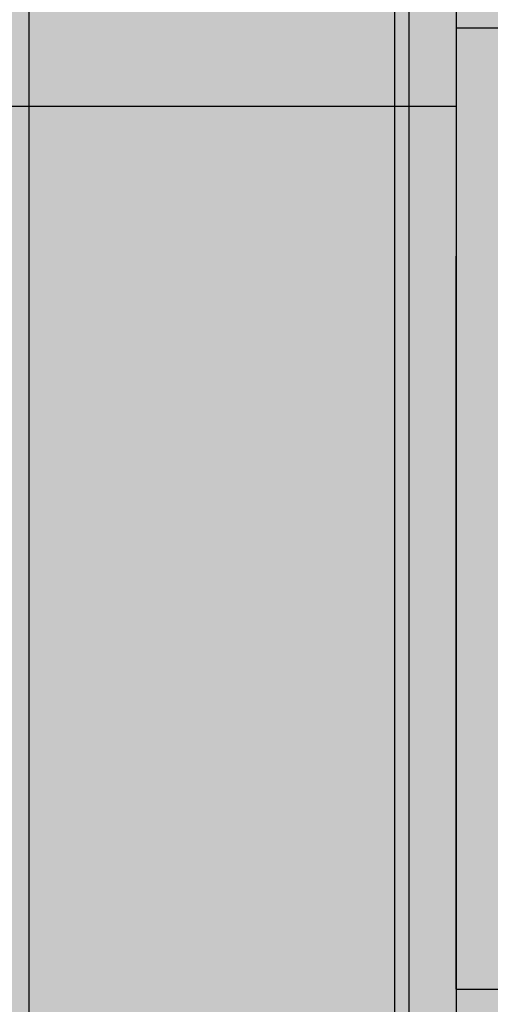
# Model space of a CAD drawing. Units: millimetres. Extents: x 131 to 845, y -20 to 1043.
# Tile 3 of 11: x 368 to 467, y 95 to 302. Entities that reach past the tile are written whole.
import ezdxf

# ---------------------------------------------------------------- set-up
doc = ezdxf.new("R2010")
doc.units = ezdxf.units.MM
doc.header["$MEASUREMENT"] = 0
for name, color, linetype, lineweight in [('A-ANNO-DIMS', 2, 'Continuous', 18), ('A-ELEV', 7, 'Continuous', 25), ('A-ELEV-PATT', 7, 'Continuous', 13), ('A-GLAZ-PATT', 143, 'Continuous', 13), ('A-WALL-PATT', 131, 'Continuous', 13)]:
    doc.layers.add(name, color=color, linetype=linetype, lineweight=lineweight)
doc.styles.get("Standard").update_dxf_attribs({"font": 'arial.ttf'})
doc.dimstyles.get("Standard").update_dxf_attribs({"dimtxt": 15, "dimasz": 10, "dimexe": 0.18, "dimexo": 0.0625, "dimgap": 5, "dimtad": 0, "dimtih": 1, "dimtoh": 1, "dimdec": 0, "dimzin": 0, "dimdsep": 46, "dimtxsty": 'Standard', "dimcen": 5, "dimadec": 0, "dimazin": 0, "dimtfac": 1, "dimtdec": 0, "dimtofl": 0, "dimtmove": 0, "dimatfit": 3, "dimfxl": 1, "dimtolj": 1, "dimtzin": 0, "dimarcsym": 0})

# ---------------------------------------------------------------- blocks, each defined once
blk = doc.blocks.new('*U5')
blk.add_line((0, 90), (0, 0))
blk = doc.blocks.new('*U6')
at = {"layer": 'A-ELEV', "color": 0, "linetype": 'ByBlock', "lineweight": -2, "transparency": 16777216, "rotation": 270}
blk.add_blockref('*U5', (369.56, 283.56), dxfattribs=at)
blk = doc.blocks.new('*D9')
at = {"layer": 'A-ANNO-DIMS', "color": 0, "lineweight": -2, "transparency": 16777216}
for p, q in [((571.05, 313.91), (561.05, 313.91)), ((581.05, 313.22), (581.05, 314.09)), ((586.05, 313.22), (586.05, 314.09)), ((596.05, 313.91), (606.05, 313.91))]:
    blk.add_line(p, q, dxfattribs=at)
at = {"layer": 'A-ANNO-DIMS', "color": 0, "transparency": 16777216}
for points in [[(571.05, 315.58), (571.05, 312.24), (581.05, 313.91)], [(596.05, 315.58), (596.05, 312.24), (586.05, 313.91)]]:
    blk.add_solid(points, dxfattribs=at)
at = {"layer": 'Defpoints', "color": 0, "transparency": 16777216}
for p in [(581.05, 313.91), (581.05, 313.16), (586.05, 313.16)]:
    blk.add_point(p, dxfattribs=at)
at = {"layer": 'A-ANNO-DIMS', "color": 0, "transparency": 16777216, "insert": (409.24, 313.91), "char_height": 15, "attachment_point": 5}
blk.add_mtext('\\A1;BALCONY RAIL PANEL 5 TYP.', dxfattribs=at)
blk = doc.blocks.new('*D14')
at = {"layer": 'A-ANNO-DIMS', "color": 0, "lineweight": -2, "transparency": 16777216}
for p, q in [((210.52, 985.67), (162.55, 985.67)), ((162.73, 975.67), (162.73, 524.4)), ((162.73, 47.81), (162.73, 499.08)), ((459.5, 37.81), (162.55, 37.81))]:
    blk.add_line(p, q, dxfattribs=at)
at = {"layer": 'A-ANNO-DIMS', "color": 0, "transparency": 16777216}
for points in [[(161.06, 975.67), (164.4, 975.67), (162.73, 985.67)], [(161.06, 47.81), (164.4, 47.81), (162.73, 37.81)]]:
    blk.add_solid(points, dxfattribs=at)
at = {"layer": 'Defpoints', "color": 0, "transparency": 16777216}
for p in [(162.73, 985.67), (210.58, 985.67), (459.56, 37.81)]:
    blk.add_point(p, dxfattribs=at)
at = {"layer": 'A-ANNO-DIMS', "color": 0, "transparency": 16777216, "insert": (162.73, 511.74), "char_height": 15, "attachment_point": 5}
blk.add_mtext('\\A1;947.9', dxfattribs=at)
blk = doc.blocks.new('*D33')
at = {"layer": 'A-ANNO-DIMS', "color": 0, "lineweight": -2, "transparency": 16777216}
for p, q in [((369.56, 283.49), (369.56, -10.22)), ((336.16, 178.37), (336.16, -10.22)), ((346.16, -10.04), (359.56, -10.04)), ((369.56, -10.04), (379.56, -10.04))]:
    blk.add_line(p, q, dxfattribs=at)
at = {"layer": 'A-ANNO-DIMS', "color": 0, "transparency": 16777216}
for points in [[(346.16, -8.37), (346.16, -11.7), (336.16, -10.04)], [(359.56, -8.37), (359.56, -11.7), (369.56, -10.04)]]:
    blk.add_solid(points, dxfattribs=at)
at = {"layer": 'Defpoints', "color": 0, "transparency": 16777216}
for p in [(369.56, 283.56), (336.16, 178.43), (369.56, -10.04)]:
    blk.add_point(p, dxfattribs=at)
at = {"layer": 'A-ANNO-DIMS', "color": 0, "transparency": 16777216, "insert": (404, -10.04), "char_height": 15, "attachment_point": 5}
blk.add_mtext('\\A1;33.4', dxfattribs=at)
blk = doc.blocks.new('*D34')
at = {"layer": 'A-ANNO-DIMS', "color": 0, "lineweight": -2, "transparency": 16777216}
for p, q in [((369.56, 283.49), (369.56, -10.22)), ((459.56, 283.49), (459.56, -10.22)), ((379.56, -10.04), (398.84, -10.04)), ((449.56, -10.04), (430.28, -10.04))]:
    blk.add_line(p, q, dxfattribs=at)
at = {"layer": 'A-ANNO-DIMS', "color": 0, "transparency": 16777216}
for points in [[(379.56, -8.37), (379.56, -11.7), (369.56, -10.04)], [(449.56, -8.37), (449.56, -11.7), (459.56, -10.04)]]:
    blk.add_solid(points, dxfattribs=at)
at = {"layer": 'Defpoints', "color": 0, "transparency": 16777216}
for p in [(369.56, 283.56), (459.56, 283.56), (459.56, -10.04)]:
    blk.add_point(p, dxfattribs=at)
at = {"layer": 'A-ANNO-DIMS', "color": 0, "transparency": 16777216, "insert": (414.56, -10.04), "char_height": 15, "attachment_point": 5}
blk.add_mtext('\\A1;90', dxfattribs=at)
blk = doc.blocks.new('*D35')
at = {"layer": 'A-ANNO-DIMS', "color": 0, "lineweight": -2, "transparency": 16777216}
for p, q in [((369.5, 763.56), (162.55, 763.56)), ((162.73, 753.56), (162.73, 536.21)), ((162.73, 293.56), (162.73, 510.9)), ((369.5, 283.56), (162.55, 283.56))]:
    blk.add_line(p, q, dxfattribs=at)
at = {"layer": 'A-ANNO-DIMS', "color": 0, "transparency": 16777216}
for points in [[(161.06, 753.56), (164.4, 753.56), (162.73, 763.56)], [(161.06, 293.56), (164.4, 293.56), (162.73, 283.56)]]:
    blk.add_solid(points, dxfattribs=at)
at = {"layer": 'Defpoints', "color": 0, "transparency": 16777216}
for p in [(162.73, 763.56), (369.56, 763.56), (369.56, 283.56)]:
    blk.add_point(p, dxfattribs=at)
at = {"layer": 'A-ANNO-DIMS', "color": 0, "transparency": 16777216, "insert": (162.73, 523.56), "char_height": 15, "attachment_point": 5}
blk.add_mtext('\\A1;480', dxfattribs=at)
blk = doc.blocks.new('*D36')
at = {"layer": 'A-ANNO-DIMS', "color": 0, "lineweight": -2, "transparency": 16777216}
for p, q in [((162.73, 333.56), (162.73, 343.56)), ((162.73, 343.56), (172.73, 343.56)), ((369.5, 323.56), (162.55, 323.56)), ((369.5, 303.56), (162.55, 303.56)), ((162.73, 293.56), (162.73, 283.56))]:
    blk.add_line(p, q, dxfattribs=at)
at = {"layer": 'A-ANNO-DIMS', "color": 0, "transparency": 16777216}
for points in [[(161.06, 333.56), (164.4, 333.56), (162.73, 323.56)], [(161.06, 293.56), (164.4, 293.56), (162.73, 303.56)]]:
    blk.add_solid(points, dxfattribs=at)
at = {"layer": 'Defpoints', "color": 0, "transparency": 16777216}
for p in [(162.73, 323.56), (369.56, 323.56), (369.56, 303.56)]:
    blk.add_point(p, dxfattribs=at)
at = {"layer": 'A-ANNO-DIMS', "color": 0, "transparency": 16777216, "insert": (188.58, 343.56), "char_height": 15, "attachment_point": 5}
blk.add_mtext('\\A1;20', dxfattribs=at)
blk = doc.blocks.new('*D37')
at = {"layer": 'A-ANNO-DIMS', "color": 0, "lineweight": -2, "transparency": 16777216}
for p, q in [((369.5, 283.56), (162.55, 283.56)), ((162.73, 273.56), (162.73, 184.6)), ((162.73, 70.31), (162.73, 159.27)), ((216.17, 60.31), (162.55, 60.31))]:
    blk.add_line(p, q, dxfattribs=at)
at = {"layer": 'A-ANNO-DIMS', "color": 0, "transparency": 16777216}
for points in [[(161.06, 273.56), (164.4, 273.56), (162.73, 283.56)], [(161.06, 70.31), (164.4, 70.31), (162.73, 60.31)]]:
    blk.add_solid(points, dxfattribs=at)
at = {"layer": 'Defpoints', "color": 0, "transparency": 16777216}
for p in [(369.56, 283.56), (162.73, 60.31), (216.23, 60.31)]:
    blk.add_point(p, dxfattribs=at)
at = {"layer": 'A-ANNO-DIMS', "color": 0, "transparency": 16777216, "insert": (162.73, 171.93), "char_height": 15, "attachment_point": 5}
blk.add_mtext('\\A1;223.24', dxfattribs=at)
blk = doc.blocks.new('*D50')
at = {"layer": 'A-ANNO-DIMS', "color": 0, "lineweight": -2, "transparency": 16777216}
for p, q in [((720.6, 488.6), (768.56, 488.6)), ((768.38, 478.6), (768.38, 287.12)), ((768.38, 70.31), (768.38, 261.79)), ((216.3, 60.31), (768.56, 60.31))]:
    blk.add_line(p, q, dxfattribs=at)
at = {"layer": 'A-ANNO-DIMS', "color": 0, "transparency": 16777216}
for points in [[(766.72, 478.6), (770.05, 478.6), (768.38, 488.6)], [(766.72, 70.31), (770.05, 70.31), (768.38, 60.31)]]:
    blk.add_solid(points, dxfattribs=at)
at = {"layer": 'Defpoints', "color": 0, "transparency": 16777216}
for p in [(720.53, 488.6), (768.38, 488.6), (216.23, 60.31)]:
    blk.add_point(p, dxfattribs=at)
at = {"layer": 'A-ANNO-DIMS', "color": 0, "transparency": 16777216, "insert": (768.38, 274.45), "char_height": 15, "attachment_point": 5}
blk.add_mtext('\\A1;428.3', dxfattribs=at)
blk = doc.blocks.new('*D72')
at = {"layer": 'A-ANNO-DIMS', "color": 0, "lineweight": -2, "transparency": 16777216}
for p, q in [((459.56, 300.1), (459.56, -10.22)), ((489.56, 300.1), (489.56, -10.22)), ((469.56, -10.04), (479.56, -10.04)), ((489.56, -10.04), (499.56, -10.04))]:
    blk.add_line(p, q, dxfattribs=at)
at = {"layer": 'A-ANNO-DIMS', "color": 0, "transparency": 16777216}
for points in [[(469.56, -8.37), (469.56, -11.7), (459.56, -10.04)], [(479.56, -8.37), (479.56, -11.7), (489.56, -10.04)]]:
    blk.add_solid(points, dxfattribs=at)
at = {"layer": 'Defpoints', "color": 0, "transparency": 16777216}
for p in [(459.56, 300.16), (489.56, 300.16), (489.56, -10.04)]:
    blk.add_point(p, dxfattribs=at)
at = {"layer": 'A-ANNO-DIMS', "color": 0, "transparency": 16777216, "insert": (515.27, -10.04), "char_height": 15, "attachment_point": 5}
blk.add_mtext('\\A1;30', dxfattribs=at)
blk = doc.blocks.new('*D75')
at = {"layer": 'A-ANNO-DIMS', "color": 0, "lineweight": -2, "transparency": 16777216}
for p, q in [((462.24, 1033.52), (452.24, 1033.52)), ((472.24, 310.22), (472.24, 1033.7)), ((489.56, 300.22), (489.56, 1033.7)), ((499.56, 1033.52), (509.56, 1033.52))]:
    blk.add_line(p, q, dxfattribs=at)
at = {"layer": 'A-ANNO-DIMS', "color": 0, "transparency": 16777216}
for points in [[(462.24, 1035.18), (462.24, 1031.85), (472.24, 1033.52)], [(499.56, 1035.18), (499.56, 1031.85), (489.56, 1033.52)]]:
    blk.add_solid(points, dxfattribs=at)
at = {"layer": 'Defpoints', "color": 0, "transparency": 16777216}
for p in [(489.56, 1033.52), (472.24, 310.16), (489.56, 300.16)]:
    blk.add_point(p, dxfattribs=at)
at = {"layer": 'A-ANNO-DIMS', "color": 0, "transparency": 16777216, "insert": (539.08, 1033.52), "char_height": 15, "attachment_point": 5}
blk.add_mtext('\\A1;17.32', dxfattribs=at)
blk = doc.blocks.new('*D99')
at = {"layer": 'A-ANNO-DIMS', "color": 0, "lineweight": -2, "transparency": 16777216}
for p, q in [((449.56, 833.53), (449.56, -10.22)), ((446.56, 818.53), (446.56, -10.22)), ((436.56, -10.04), (426.56, -10.04)), ((459.56, -10.04), (469.56, -10.04))]:
    blk.add_line(p, q, dxfattribs=at)
at = {"layer": 'A-ANNO-DIMS', "color": 0, "transparency": 16777216}
for points in [[(436.56, -8.37), (436.56, -11.7), (446.56, -10.04)], [(459.56, -8.37), (459.56, -11.7), (449.56, -10.04)]]:
    blk.add_solid(points, dxfattribs=at)
at = {"layer": 'Defpoints', "color": 0, "transparency": 16777216}
for p in [(449.56, 833.6), (446.56, 818.6), (449.56, -10.04)]:
    blk.add_point(p, dxfattribs=at)
at = {"layer": 'A-ANNO-DIMS', "color": 0, "transparency": 16777216, "insert": (479.47, -10.04), "char_height": 15, "attachment_point": 5}
blk.add_mtext('\\A1;3', dxfattribs=at)

msp = doc.modelspace()

# ---------------------------------------------------------------- hatches: boundary and pattern name
at = {"layer": 'A-ELEV-PATT', "transparency": 33554681}
h = msp.add_hatch(color=256, dxfattribs=at)
h.set_gradient(color1=(147, 149, 152), color2=(192, 192, 192), name='CURVED')
h.paths.add_polyline_path([(369.5586, 743.5561), (369.5586, 723.5561), (459.5586, 723.5561), (459.5586, 743.5561)])
h.paths.add_polyline_path([(369.5586, 703.5561), (369.5586, 683.5561), (459.5586, 683.5561), (459.5586, 703.5561)])
h.paths.add_polyline_path([(459.5586, 643.5561), (459.5586, 663.5561), (369.5586, 663.5561), (369.5586, 643.5561)])
h.paths.add_polyline_path([(459.5586, 603.5561), (459.5586, 623.5561), (369.5586, 623.5561), (369.5586, 603.5561)])
h.paths.add_polyline_path([(369.5586, 583.5561), (369.5586, 563.5561), (459.5586, 563.5561), (459.5586, 583.5561)])
h.paths.add_polyline_path([(369.5586, 543.5561), (369.5586, 523.5561), (459.5586, 523.5561), (459.5586, 543.5561)])
h.paths.add_polyline_path([(459.5586, 483.5561), (459.5586, 488.5953), (412.6606, 488.5953), (412.6606, 498.5953), (409.6606, 498.5953), (409.6606, 503.5561), (369.5586, 503.5561), (369.5586, 483.5561)])
h.paths.add_polyline_path([(369.5586, 463.5561), (369.5586, 443.5561), (459.5586, 443.5561), (459.5586, 463.5561)])
h.paths.add_polyline_path([(369.5586, 423.5561), (369.5586, 403.5561), (459.5586, 403.5561), (459.5586, 423.5561)])
h.paths.add_polyline_path([(369.5586, 383.5561), (369.5586, 363.5561), (459.5586, 363.5561), (459.5586, 383.5561)])
h.paths.add_polyline_path([(369.5586, 343.5561), (369.5586, 323.5561), (459.5586, 323.5561), (459.5586, 343.5561)])
h.paths.add_polyline_path([(369.5586, 303.5561), (369.5586, 283.5561), (459.5586, 283.5561), (459.5586, 303.5561)])
h = msp.add_hatch(color=256, dxfattribs=at)
h.set_gradient(color1=(79, 2, 22), color2=(153, 133, 76), name='SPHERICAL')
h.paths.add_polyline_path([(459.5586, 310.1596), (459.5586, 300.1596), (489.5586, 300.1596), (472.2381, 310.1596)])
h.paths.add_polyline_path([(658.8842, 312.6596), (628.8842, 312.6596), (650.5349, 300.1596), (680.5349, 300.1596)])
h = msp.add_hatch(color=256, dxfattribs=at)
h.set_gradient(color1=(255, 255, 255), color2=(199, 200, 202), name='INVSPHERICAL')
h.paths.add_polyline_path([(489.5586, 300.1596), (459.5586, 300.1596), (459.5586, 252.07), (459.5586, 97.8131), (489.5586, 97.8131)])
h.paths.add_polyline_path([(680.5349, 300.1596), (650.5349, 300.1596), (650.5349, 97.8131), (680.5349, 97.8131)])
h.paths.add_polyline_path([(658.5215, 82.8131), (459.5586, 82.8131), (459.5586, 67.8131), (658.5215, 67.8131)])
h.paths.add_polyline_path([(663.9762, 52.8131), (459.5586, 52.8131), (459.5586, 37.8131), (663.9762, 37.8131)])
h.paths.add_polyline_path([(680.5349, 97.8131), (650.5349, 97.8131), (658.5215, 82.8131), (658.5215, 67.8131), (661.2489, 60.3131), (680.5349, 60.3131)])
at = {"layer": 'A-GLAZ-PATT'}
h = msp.add_hatch(color=256, dxfattribs=at)
h.dxf.hatch_style = 1
h.paths.add_polyline_path([(658.8074, 488.5953), (628.8842, 488.5953), (628.8842, 312.6596), (658.8842, 312.6596)])
h.paths.add_polyline_path([(650.5349, 97.8131), (459.5586, 97.8131), (459.5586, 82.8131), (658.5215, 82.8131)])
h.paths.add_polyline_path([(658.5215, 67.8131), (459.5586, 67.8131), (459.5586, 52.8131), (663.9762, 52.8131)])
at = {"layer": 'A-WALL-PATT'}
h = msp.add_hatch(color=256, dxfattribs=at)
h.dxf.hatch_style = 1
h.paths.add_polyline_path([(449.5586, 833.5953), (451.6297, 835.6663), (451.6297, 885.6663), (466.6297, 885.6663), (466.6297, 891.3345), (330.6595, 891.3345), (330.6595, 856.8345), (292.1595, 856.8345), (292.1595, 798.4332), (336.1595, 798.4332), (336.1595, 178.4332), (246.1595, 178.4332), (246.1595, 798.4332), (290.1595, 798.4332), (290.1595, 856.8345), (259.6595, 856.8345), (255.6595, 860.8345), (255.6595, 927.8345), (290.1595, 927.8345), (290.1595, 960.6663), (216.2327, 960.6663), (216.2327, 60.3131), (459.5586, 60.3131), (459.5586, 97.8131), (459.5586, 252.07), (459.5586, 283.5561), (369.5586, 283.5561), (369.5586, 763.5561), (439.5586, 763.5561), (439.5586, 778.6714), (439.5586, 793.5953), (439.5586, 796.5953), (441.5586, 798.5953), (444.5586, 798.5953), (444.5586, 813.5953), (444.5586, 816.5953), (446.5586, 818.5953), (449.5586, 818.5953)])
h.paths.add_polyline_path([(466.6297, 960.6663), (292.1595, 960.6663), (292.1595, 927.8345), (326.6595, 927.8345), (330.6595, 923.8345), (330.6595, 893.3345), (466.6297, 893.3345)], flags=17)
h.paths.add_polyline_path([(720.5349, 813.5953), (720.5349, 818.5953), (710.5349, 818.5953), (449.5586, 818.5953), (446.5586, 818.5953), (444.5586, 816.5953), (444.5586, 813.5953), (444.5586, 798.5953), (705.5349, 798.5953), (705.5349, 513.5953), (705.5349, 498.5953), (680.5349, 498.5953), (680.5349, 488.5953), (705.5349, 488.5953), (720.5349, 488.5953), (720.5349, 513.5953)])
h.paths.add_polyline_path([(680.5349, 498.5953), (412.6606, 498.5953), (412.6606, 488.5953), (680.5349, 488.5953)])

# ---------------------------------------------------------------- linework, layer by layer
at = {"layer": 'A-ELEV'}
for p, q in [((369.5586, 763.5561), (369.5586, 283.5561)), ((459.5586, 488.5953), (459.5586, 252.07)), ((459.5586, 300.1596), (489.5586, 300.1596)), ((459.5586, 97.8131), (459.5586, 252.07)), ((459.5586, 97.8131), (650.5349, 97.8131)), ((459.5586, 97.8131), (459.5586, 37.8131))]:
    msp.add_line(p, q, dxfattribs=at)

# ---------------------------------------------------------------- block references
msp.add_blockref('*U6', (0, 0), dxfattribs=at)

# ---------------------------------------------------------------- dimensions: what is measured, and where the dimension line sits
at = {"layer": 'A-ANNO-DIMS'}
for base, p1, p2, override, picture, middle in [((489.5586, 1033.5163), (472.2381, 310.1596), (489.5586, 300.1596), {"dimdec": 2, "dimlfac": 1, "dimrnd": 0, "dimzin": 0, "dimdsep": 46, "dimlunit": 2}, '*D75', (539.0845, 1033.5163)), ((449.5586, -10.0369), (446.5586, 818.5953), (449.5586, 833.5953), {"dimdec": 0, "dimlfac": 1, "dimrnd": 0, "dimzin": 0, "dimdsep": 46, "dimlunit": 2}, '*D99', (479.4699, -10.0369)), ((489.5586, -10.0369), (459.5586, 300.1596), (489.5586, 300.1596), {"dimdec": 0, "dimlfac": 1, "dimrnd": 0, "dimzin": 0, "dimdsep": 46, "dimlunit": 2}, '*D72', (515.2714, -10.0369)), ((369.5586, -10.0369), (336.1595, 178.4332), (369.5586, 283.5561), {"dimdec": 1, "dimlfac": 1, "dimrnd": 0, "dimzin": 0, "dimdsep": 46, "dimlunit": 2}, '*D33', (404.0044, -10.0369)), ((459.5586, -10.0369), (369.5586, 283.5561), (459.5586, 283.5561), {"dimdec": 0, "dimlfac": 1, "dimrnd": 0, "dimzin": 0, "dimdsep": 46, "dimlunit": 2}, '*D34', (414.5586, -10.0369))]:
    dim = msp.add_linear_dim(base=base, p1=p1, p2=p2, dimstyle='Standard', override=override, dxfattribs=at)
    dim.commit()
    dim.dimension.update_dxf_attribs({"geometry": picture, "text_midpoint": middle})
for base, p1, p2, override, picture, middle in [((162.7317, 985.6663), (459.5586, 37.8131), (210.5817, 985.6663), {"dimdec": 1, "dimlfac": 1, "dimrnd": 0, "dimzin": 0, "dimdsep": 46, "dimlunit": 2}, '*D14', (162.7317, 511.7397)), ((162.7317, 763.5561), (369.5586, 283.5561), (369.5586, 763.5561), {"dimdec": 0, "dimlfac": 1, "dimrnd": 0, "dimzin": 0, "dimdsep": 46, "dimlunit": 2}, '*D35', (162.7317, 523.5561)), ((768.3849, 488.5953), (216.2327, 60.3131), (720.5349, 488.5953), {"dimdec": 1, "dimlfac": 1, "dimrnd": 0, "dimzin": 0, "dimdsep": 46, "dimlunit": 2}, '*D50', (768.3849, 274.4542)), ((162.7317, 323.5561), (369.5586, 303.5561), (369.5586, 323.5561), {"dimdec": 0, "dimlfac": 1, "dimrnd": 0, "dimzin": 0, "dimdsep": 46, "dimlunit": 2}, '*D36', (188.5775, 343.5561)), ((162.7317, 60.3131), (369.5586, 283.5561), (216.2327, 60.3131), {"dimdec": 2, "dimlfac": 1, "dimrnd": 0, "dimzin": 0, "dimdsep": 46, "dimlunit": 2}, '*D37', (162.7317, 171.9346))]:
    dim = msp.add_linear_dim(base=base, p1=p1, p2=p2, angle=90, dimstyle='Standard', override=override, dxfattribs=at)
    dim.commit()
    dim.dimension.update_dxf_attribs({"geometry": picture, "text_midpoint": middle})
dim = msp.add_linear_dim(base=(581.0467, 313.9096), p1=(586.0467, 313.1596), p2=(581.0467, 313.1596), angle=180, text='BALCONY RAIL PANEL <> TYP.', dimstyle='Standard', override={"dimdec": 0, "dimrnd": 0, "dimzin": 0, "dimlunit": 2}, dxfattribs=at)
dim.commit()
dim.dimension.update_dxf_attribs({"geometry": '*D9', "text_midpoint": (409.2391, 313.9096)})

doc.saveas('drawing.dxf')
